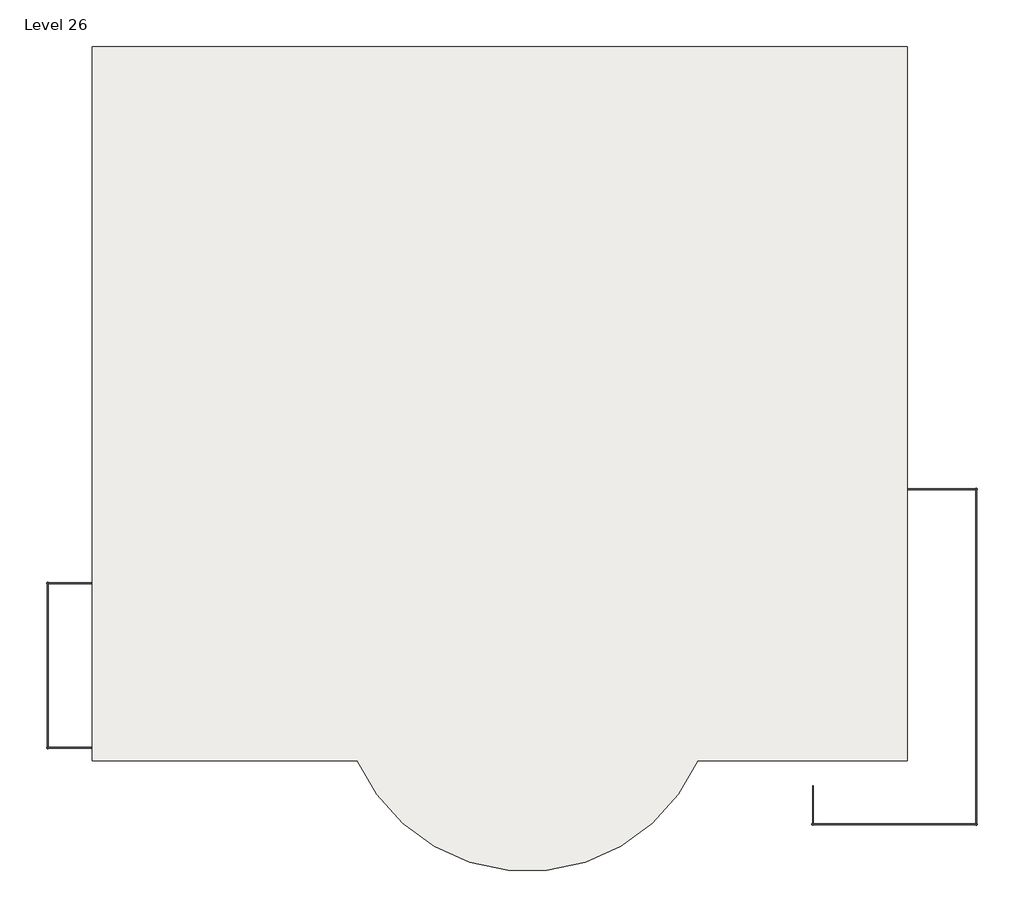
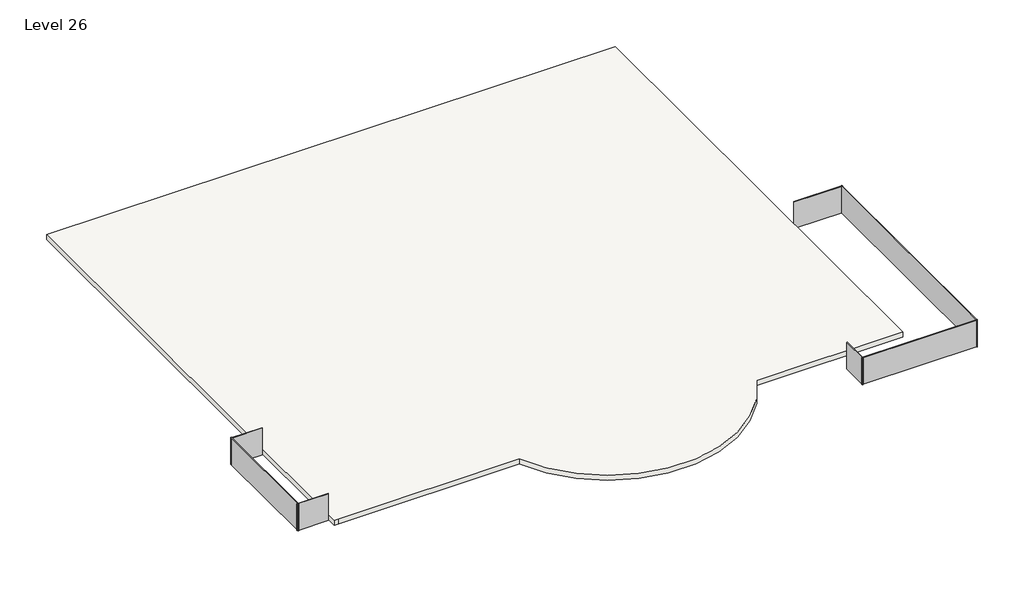
# One storey: 7 plates, 1 slab.
"""IFC4 building model written with IfcOpenShell, lengths in millimetres."""

from ifc_helpers import new_model, si_unit, point, frame, frame_2d, origin, place, context, project, spatial, polyline, circle_curve, trimmed, segment, composite_curve, outline, extrude, transform, mapped, element, save
from components import system_panel_glazed_7d767388, system_panel_glazed_a5f349e9, system_panel_glazed_f6fb2dd6, system_panel_glazed_8bf14ce2, system_panel_glazed_decb64e8, system_panel_glazed_5b5c8ea9

model = new_model("IFC4")

# Units and contexts
model_context = context("Model", 3, world=origin())
ifc_project = project(units=[si_unit("LENGTHUNIT", "METRE", prefix="MILLI")], contexts=[model_context])

# Site, building, storey
site = spatial("IfcSite", under=ifc_project)
building = spatial("IfcBuilding", under=site)
storey = spatial("IfcBuildingStorey", under=building, Name="Level 26", Elevation=42367.2)

# Plates
placement = place(None, origin())
system_panel_glazed_shape = system_panel_glazed_7d767388(model_context)
element("IfcPlate", 1, ObjectType="System Panel : Glazed", at=placement, inside=storey, context=model_context, shape_type="MappedRepresentation", body=[
    mapped(system_panel_glazed_shape, transform((-17306.4505427, -8690.0239591, 42367.2), x_axis=(-1.0, 0.0, 0.0), y_axis=(0.0, -1.0, 0.0), z_axis=(0.0, 0.0, 1.0))),
])
element("IfcPlate", 2, ObjectType="System Panel : Glazed", at=placement, inside=storey, context=model_context, shape_type="MappedRepresentation", body=[
    mapped(system_panel_glazed_shape, transform((-17306.4505427, -13712.8739591, 42367.2), x_axis=(1.0, 0.0, 0.0), y_axis=(0.0, 1.0, 0.0), z_axis=(0.0, 0.0, 1.0))),
])
system_panel_glazed_2_shape = system_panel_glazed_a5f349e9(model_context)
element("IfcPlate", 3, ObjectType="System Panel : Glazed", at=placement, inside=storey, context=model_context, shape_type="MappedRepresentation", body=[
    mapped(system_panel_glazed_2_shape, transform((-17979.5505427, -11201.4489591, 42367.2), x_axis=(0.0, -1.0, 0.0), y_axis=(1.0, 0.0, 0.0), z_axis=(0.0, 0.0, 1.0))),
])
system_panel_glazed_3_shape = system_panel_glazed_f6fb2dd6(model_context)
element("IfcPlate", 4, ObjectType="System Panel : Glazed", at=placement, inside=storey, context=model_context, shape_type="MappedRepresentation", body=[
    mapped(system_panel_glazed_3_shape, transform((5101.1464352, -15423.3278294, 42367.2), x_axis=(0.0, -1.0, 0.0), y_axis=(1.0, 0.0, 0.0), z_axis=(0.0, 0.0, 1.0))),
])
system_panel_glazed_4_shape = system_panel_glazed_8bf14ce2(model_context)
element("IfcPlate", 5, ObjectType="System Panel : Glazed", at=placement, inside=storey, context=model_context, shape_type="MappedRepresentation", body=[
    mapped(system_panel_glazed_4_shape, transform((7596.6964352, -16020.2278294, 42367.2), x_axis=(1.0, 0.0, 0.0), y_axis=(0.0, 1.0, 0.0), z_axis=(0.0, 0.0, 1.0))),
])
system_panel_glazed_5_shape = system_panel_glazed_decb64e8(model_context)
element("IfcPlate", 6, ObjectType="System Panel : Glazed", at=placement, inside=storey, context=model_context, shape_type="MappedRepresentation", body=[
    mapped(system_panel_glazed_5_shape, transform((10092.2464352, -10940.2278294, 42367.2), x_axis=(0.0, 1.0, 0.0), y_axis=(-1.0, 0.0, 0.0), z_axis=(0.0, 0.0, 1.0))),
])
system_panel_glazed_6_shape = system_panel_glazed_5b5c8ea9(model_context)
element("IfcPlate", 7, ObjectType="System Panel : Glazed", at=placement, inside=storey, context=model_context, shape_type="MappedRepresentation", body=[
    mapped(system_panel_glazed_6_shape, transform((9038.1464352, -5860.2278294, 42367.2), x_axis=(-1.0, 0.0, 0.0), y_axis=(0.0, -1.0, 0.0), z_axis=(0.0, 0.0, 1.0))),
])

# Slab
element("IfcSlab", 8, ObjectType="9\"", at=placement, inside=storey, context=model_context, shape_type="SweptSolid", body=[
    extrude(outline(composite_curve([segment(polyline([(-16607.9505427, 7462.0454004), (7979.2494573, 7462.0454004), (7979.2494573, -14077.1545996), (1652.8739931, -14077.1545996)]), True, "CONTINUOUS"), segment(trimmed(circle_curve(frame_2d((-3476.1505427, -11787.4387998)), 5616.9111737), [point((1652.8739931, -14077.1545996))], [point((-8605.1750786, -14077.1545996))], False, "CARTESIAN"), True, "CONTINUOUS"), segment(polyline([(-8605.1750786, -14077.1545996), (-16404.7505427, -14077.1545996), (-16607.9505427, -14077.1545996), (-16607.9505427, 7462.0454004)]), True, "CONTINUOUS")], self_intersect=False)), frame((0.0, 0.0, 42370.3192887), z_axis=(0.0, 0.0, 1.0), x_axis=(1.0, 0.0, 0.0)), (0.0, 0.0, 1.0), 228.6),
])

save(model, "model.ifc")

# Revit data of these elements
# Type "System Panel : Glazed"
#   Construction Type Id = "GSP4R"
#   Analytic Construction = "1/8 in Pilkington single glazing"
#   Visual Light Transmittance = 0.9
#   Solar Heat Gain Coefficient = 0.86
#   Heat Transfer Coefficient (U) = 1.18115 BTU/(h·ft²·°F)
# Type "9\""
#   Assembly Code = "B1010"
#   Function = 0
#   Layers, outside or top first: 0' - 9" no material (function 1)
# Elements 1, 2, 3, 4, 5, 6, 7 (IfcPlate, "System Panel : Glazed")
#   Phase Created = New Construction
#   Materials on its faces: "Glass"
# Element 8 (IfcSlab, "9\"")
#   built-in parameter 1001955 = 1.5708 (stored number, unit not read)
#   Height Offset From Level = 0' - 9.12281"
#   Phase Created = New Construction
#   Materials on its faces: "Default Floor"
# Materials
#   "Glass": class "Glass", colour RGB 0 128 192, transparency 0.75, Description = "Soda Lime Glass", Cost = 0
#   "Default Floor": colour RGB 128 128 128, transparency 0
